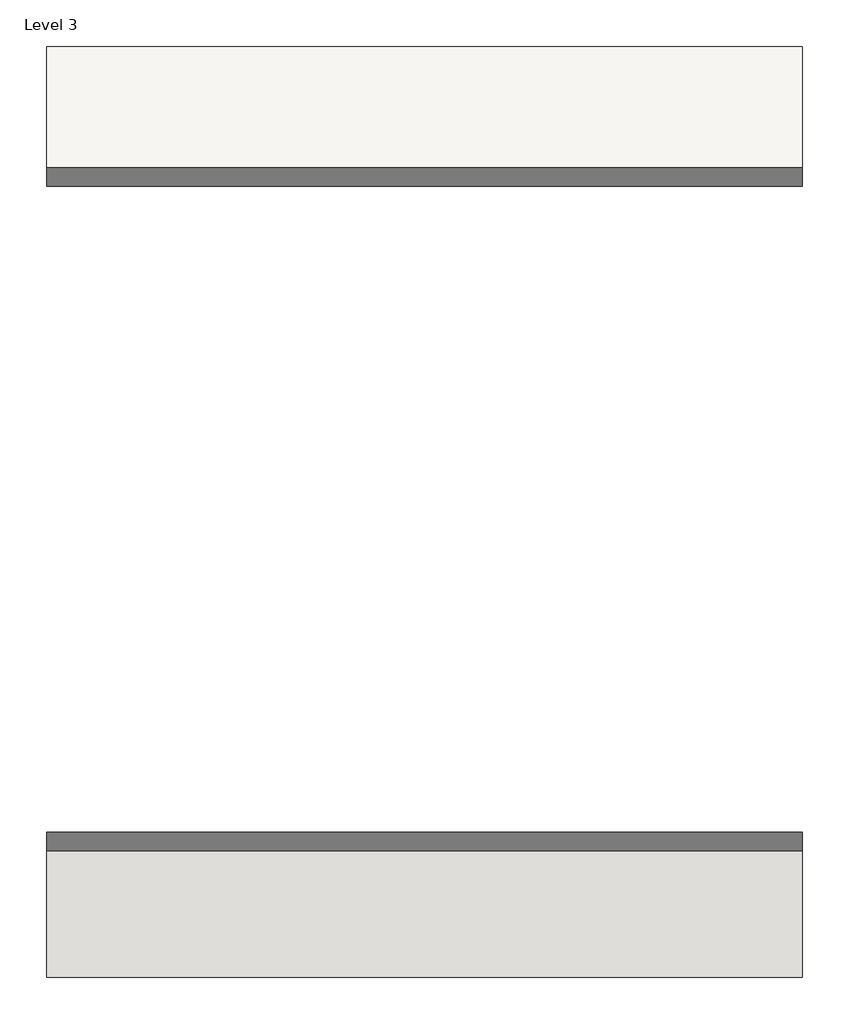
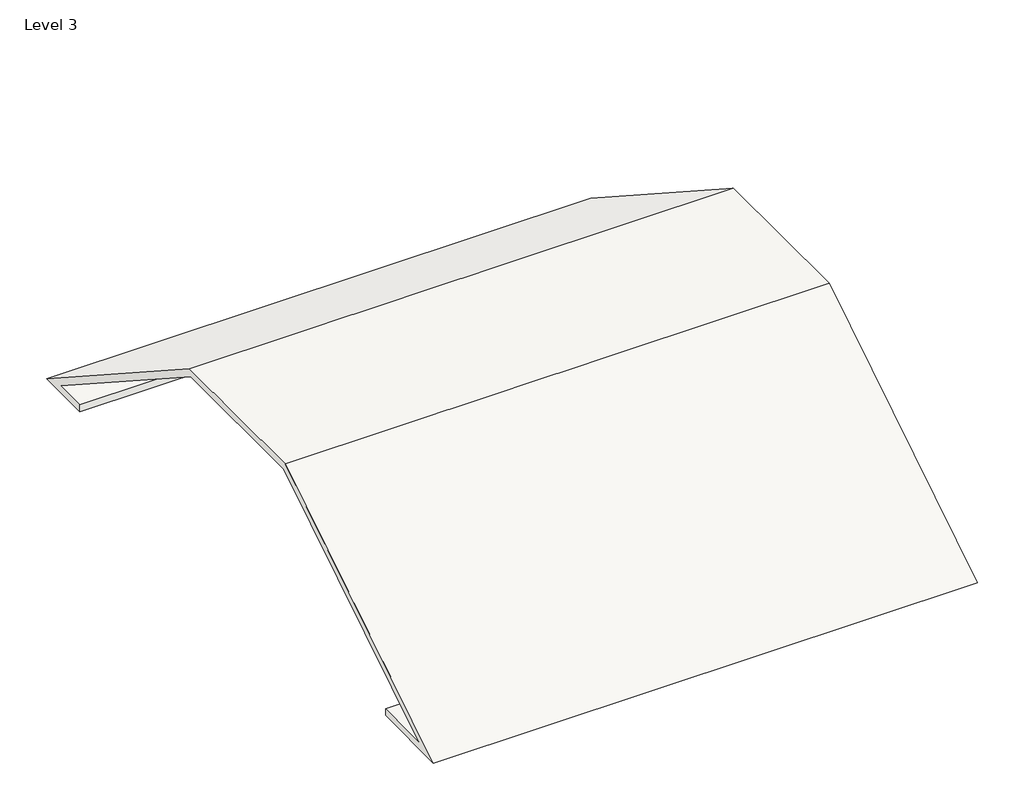
# One storey: 1 roof.
"""IFC4 building model written with IfcOpenShell, lengths in millimetres."""

from ifc_helpers import new_model, si_unit, frame, origin, place, context, project, spatial, polyline, outline, extrude, element, save

model = new_model("IFC4")

# Units and contexts
model_context = context("Model", 3, world=origin())
ifc_project = project(units=[si_unit("LENGTHUNIT", "METRE", prefix="MILLI")], contexts=[model_context])

# Site, building, storey
site = spatial("IfcSite", under=ifc_project)
building = spatial("IfcBuilding", under=site)
storey = spatial("IfcBuildingStorey", under=building, Name="Level 3", Elevation=6400.8)

# Roof
placement = place(None, origin())
element("IfcRoof", 1, ObjectType="Generic - 12\"", at=placement, inside=storey, context=model_context, shape_type="SweptSolid", body=[
    extrude(outline(polyline([(-2449.8776789, 6400.8), (-4204.7508603, 6400.8), (1233.1223211, 9798.7602906), (4738.3223211, 9798.7602906), (9970.7223211, 6400.8), (8751.5223211, 6400.8), (8751.5223211, 6553.2), (9456.2285435, 6553.2), (4693.1793845, 9646.3602906), (1276.8223179, 9646.3602906), (-3673.2688991, 6553.2), (-2449.8776789, 6553.2), (-2449.8776789, 6400.8)])), frame((-5844.0328791, 0.0, 0.0), z_axis=(1.0, 0.0, 0.0), x_axis=(0.0, 1.0, 0.0)), (0.0, 0.0, 1.0), 11506.2),
])

save(model, "model.ifc")

# Revit data of these elements
# Type "Generic - 12\""
#   Assembly Code = "B1020"
#   Layers, outside or top first: 0' - 6" "roofing material 1'" (function 1)
# Element 1 (IfcRoof, "Generic - 12\"")
#   built-in parameter 1001710 = 33615
#   Phase Created = New Construction
#   Materials on its faces: "roofing material 1'"
# Materials
#   "roofing material 1'": class "Generic", colour RGB 120 120 120, transparency 0, Cost = 0
